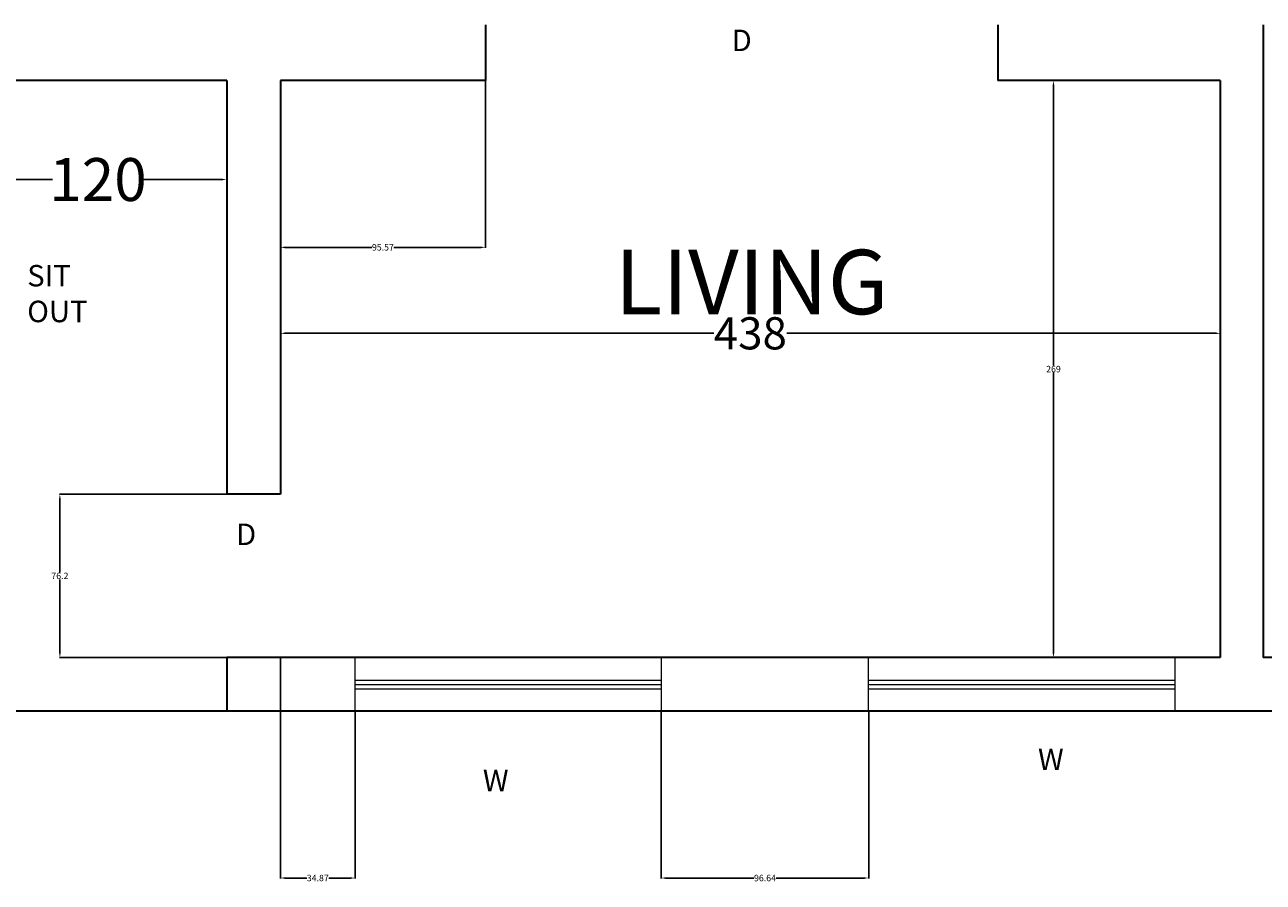
# Model space of a CAD drawing. Units: centimetres. Extents: x -121 to 3851, y -16 to 1180.
# Tile 2 of 16: x 381 to 958, y -16 to 384. Entities that reach past the tile are written whole.
import ezdxf

# ---------------------------------------------------------------- set-up
doc = ezdxf.new("R2010")
doc.units = ezdxf.units.CM
doc.header["$MEASUREMENT"] = 0
for name, color, linetype, lineweight in [('A-ANNO-DIMS', 2, 'Continuous', 18), ('A-ANNO-IDEN', 3, 'Continuous', 13), ('A-AREA-IDEN', 3, 'Continuous', 18), ('A-GLAZ', 4, 'Continuous', 18), ('A-WALL', 7, 'Continuous', 35)]:
    doc.layers.add(name, color=color, linetype=linetype, lineweight=lineweight)
doc.styles.get("Standard").update_dxf_attribs({"font": 'arial.ttf'})
doc.dimstyles.get("Standard").update_dxf_attribs({"dimtxt": 3, "dimasz": 2, "dimexe": 0.18, "dimexo": 0.0625, "dimgap": 0.09, "dimtad": 0, "dimtih": 1, "dimtoh": 1, "dimdec": 0, "dimzin": 0, "dimdsep": 46, "dimtxsty": 'Standard', "dimcen": 0.09, "dimadec": 0, "dimazin": 0, "dimtfac": 1, "dimtdec": 0, "dimtofl": 0, "dimtmove": 0, "dimatfit": 3, "dimfxl": 1, "dimtolj": 1, "dimtzin": 0, "dimarcsym": 0})

# ---------------------------------------------------------------- blocks, each defined once
blk = doc.blocks.new('*D8')
at = {"layer": 'A-ANNO-DIMS', "color": 0, "lineweight": -2, "transparency": 16777216}
for p, q in [((355.04, 281.89), (355.04, 312.04)), ((357.04, 311.86), (393.83, 311.86)), ((473.04, 311.86), (436.25, 311.86)), ((475.04, 281.89), (475.04, 312.04))]:
    blk.add_line(p, q, dxfattribs=at)
at = {"layer": 'A-ANNO-DIMS', "color": 0, "transparency": 16777216}
for points in [[(357.04, 312.19), (357.04, 311.52), (355.04, 311.86)], [(473.04, 312.19), (473.04, 311.52), (475.04, 311.86)]]:
    blk.add_solid(points, dxfattribs=at)
at = {"layer": 'Defpoints', "color": 0, "transparency": 16777216}
for p in [(475.04, 311.86), (355.04, 281.82), (475.04, 281.82)]:
    blk.add_point(p, dxfattribs=at)
at = {"layer": 'A-ANNO-DIMS', "color": 0, "transparency": 16777216, "insert": (415.04, 311.86), "char_height": 3, "attachment_point": 5}
blk.add_mtext('\\A1;{\\H6.66667x;120}', dxfattribs=at)
blk = doc.blocks.new('*D10')
at = {"layer": 'A-ANNO-DIMS', "color": 0, "lineweight": -2, "transparency": 16777216}
for p, q in [((500.04, 198.01), (500.04, 240.36)), ((502.04, 240.18), (702.06, 240.18)), ((936.04, 240.18), (736.02, 240.18)), ((938.04, 198.01), (938.04, 240.36))]:
    blk.add_line(p, q, dxfattribs=at)
at = {"layer": 'A-ANNO-DIMS', "color": 0, "transparency": 16777216}
for points in [[(502.04, 240.52), (502.04, 239.85), (500.04, 240.18)], [(936.04, 240.52), (936.04, 239.85), (938.04, 240.18)]]:
    blk.add_solid(points, dxfattribs=at)
at = {"layer": 'Defpoints', "color": 0, "transparency": 16777216}
for p in [(938.04, 240.18), (500.04, 197.94), (938.04, 197.94)]:
    blk.add_point(p, dxfattribs=at)
at = {"layer": 'A-ANNO-DIMS', "color": 0, "transparency": 16777216, "insert": (719.04, 240.18), "char_height": 3, "attachment_point": 5}
blk.add_mtext('\\A1;{\\H5x;438}', dxfattribs=at)
blk = doc.blocks.new('WIN-143CM')
for p, q in [((0, 14.5), (142.63, 14.5)), ((0, 12.5), (142.63, 12.5)), ((0, 10.5), (142.63, 10.5))]:
    blk.add_line(p, q)
blk.add_lwpolyline([(0, 25), (142.63, 25), (142.63, 0), (0, 0)], close=True)
blk = doc.blocks.new('*D44')
at = {"layer": 'A-ANNO-DIMS', "color": 0, "lineweight": -2, "transparency": 16777216}
for p, q in [((474.98, 165.21), (397.11, 165.21)), ((397.29, 163.21), (397.29, 128.73)), ((397.29, 91.01), (397.29, 125.49)), ((474.98, 89.01), (397.11, 89.01))]:
    blk.add_line(p, q, dxfattribs=at)
at = {"layer": 'A-ANNO-DIMS', "color": 0, "transparency": 16777216}
for points in [[(396.95, 163.21), (397.62, 163.21), (397.29, 165.21)], [(396.95, 91.01), (397.62, 91.01), (397.29, 89.01)]]:
    blk.add_solid(points, dxfattribs=at)
at = {"layer": 'Defpoints', "color": 0, "transparency": 16777216}
for p in [(397.29, 165.21), (475.04, 165.21), (475.04, 89.01)]:
    blk.add_point(p, dxfattribs=at)
at = {"layer": 'A-ANNO-DIMS', "color": 0, "transparency": 16777216, "insert": (397.29, 127.11), "char_height": 3, "attachment_point": 5}
blk.add_mtext('\\A1;76.2', dxfattribs=at)
blk = doc.blocks.new('*D46')
at = {"layer": 'A-ANNO-DIMS', "color": 0, "lineweight": -2, "transparency": 16777216}
for p, q in [((500.04, 357.95), (500.04, 280.08)), ((595.61, 357.95), (595.61, 280.08)), ((502.04, 280.26), (542.67, 280.26)), ((593.61, 280.26), (552.98, 280.26))]:
    blk.add_line(p, q, dxfattribs=at)
at = {"layer": 'A-ANNO-DIMS', "color": 0, "transparency": 16777216}
for points in [[(502.04, 280.6), (502.04, 279.93), (500.04, 280.26)], [(593.61, 280.6), (593.61, 279.93), (595.61, 280.26)]]:
    blk.add_solid(points, dxfattribs=at)
at = {"layer": 'Defpoints', "color": 0, "transparency": 16777216}
for p in [(500.04, 358.01), (595.61, 358.01), (500.04, 280.26)]:
    blk.add_point(p, dxfattribs=at)
at = {"layer": 'A-ANNO-DIMS', "color": 0, "transparency": 16777216, "insert": (547.82, 280.26), "char_height": 3, "attachment_point": 5}
blk.add_mtext('\\A1;95.57', dxfattribs=at)
blk = doc.blocks.new('*D47')
at = {"layer": 'A-ANNO-DIMS', "color": 0, "lineweight": -2, "transparency": 16777216}
for p, q in [((937.98, 358.01), (860.11, 358.01)), ((860.29, 356.01), (860.29, 225.14)), ((860.29, 91.01), (860.29, 221.89)), ((937.98, 89.01), (860.11, 89.01))]:
    blk.add_line(p, q, dxfattribs=at)
at = {"layer": 'A-ANNO-DIMS', "color": 0, "transparency": 16777216}
for points in [[(859.95, 356.01), (860.62, 356.01), (860.29, 358.01)], [(859.95, 91.01), (860.62, 91.01), (860.29, 89.01)]]:
    blk.add_solid(points, dxfattribs=at)
at = {"layer": 'Defpoints', "color": 0, "transparency": 16777216}
for p in [(860.29, 358.01), (938.04, 358.01), (938.04, 89.01)]:
    blk.add_point(p, dxfattribs=at)
at = {"layer": 'A-ANNO-DIMS', "color": 0, "transparency": 16777216, "insert": (860.29, 223.51), "char_height": 3, "attachment_point": 5}
blk.add_mtext('\\A1;269', dxfattribs=at)
blk = doc.blocks.new('*D48')
at = {"layer": 'A-ANNO-DIMS', "color": 0, "lineweight": -2, "transparency": 16777216}
for p, q in [((500.04, 88.95), (500.04, -13.92)), ((534.91, 63.95), (534.91, -13.92)), ((502.04, -13.74), (512.32, -13.74)), ((532.91, -13.74), (522.62, -13.74))]:
    blk.add_line(p, q, dxfattribs=at)
at = {"layer": 'A-ANNO-DIMS', "color": 0, "transparency": 16777216}
for points in [[(502.04, -13.4), (502.04, -14.07), (500.04, -13.74)], [(532.91, -13.4), (532.91, -14.07), (534.91, -13.74)]]:
    blk.add_solid(points, dxfattribs=at)
at = {"layer": 'Defpoints', "color": 0, "transparency": 16777216}
for p in [(500.04, 89.01), (534.91, 64.01), (500.04, -13.74)]:
    blk.add_point(p, dxfattribs=at)
at = {"layer": 'A-ANNO-DIMS', "color": 0, "transparency": 16777216, "insert": (517.47, -13.74), "char_height": 3, "attachment_point": 5}
blk.add_mtext('\\A1;34.87', dxfattribs=at)
blk = doc.blocks.new('*D49')
at = {"layer": 'A-ANNO-DIMS', "color": 0, "lineweight": -2, "transparency": 16777216}
for p, q in [((677.54, 63.95), (677.54, -13.92)), ((774.18, 63.95), (774.18, -13.92)), ((679.54, -13.74), (720.71, -13.74)), ((772.18, -13.74), (731, -13.74))]:
    blk.add_line(p, q, dxfattribs=at)
at = {"layer": 'A-ANNO-DIMS', "color": 0, "transparency": 16777216}
for points in [[(679.54, -13.4), (679.54, -14.07), (677.54, -13.74)], [(772.18, -13.4), (772.18, -14.07), (774.18, -13.74)]]:
    blk.add_solid(points, dxfattribs=at)
at = {"layer": 'Defpoints', "color": 0, "transparency": 16777216}
for p in [(677.54, 64.01), (774.18, 64.01), (774.18, -13.74)]:
    blk.add_point(p, dxfattribs=at)
at = {"layer": 'A-ANNO-DIMS', "color": 0, "transparency": 16777216, "insert": (725.86, -13.74), "char_height": 3, "attachment_point": 5}
blk.add_mtext('\\A1;96.64', dxfattribs=at)

msp = doc.modelspace()

# ---------------------------------------------------------------- linework, layer by layer
at = {"layer": 'A-WALL'}
for p, q in [((595.6084, 384.0141), (595.6084, 358.0141)), ((834.382, 384.0141), (834.382, 358.0141)), ((958.0382, 384.0141), (958.0382, 89.0141)), ((475.0382, 358.0141), (65.0382, 358.0141)), ((475.0382, 358.0141), (475.0382, 165.2103)), ((500.0382, 358.0141), (500.0382, 165.2103)), ((595.6084, 358.0141), (500.0382, 358.0141)), ((938.0382, 358.0141), (834.382, 358.0141)), ((938.0382, 358.0141), (938.0382, 89.0141)), ((500.0382, 165.2103), (475.0382, 165.2103)), ((500.0382, 89.0141), (475.0382, 89.0141)), ((475.0382, 89.0141), (475.0382, 64.0141)), ((938.0382, 89.0141), (500.0382, 89.0141)), ((1396.0382, 89.0141), (958.0382, 89.0141)), ((1421.0382, 64.0141), (65.0382, 64.0141))]:
    msp.add_line(p, q, dxfattribs=at)

# ---------------------------------------------------------------- block references
at = {"layer": 'A-GLAZ'}
for p in [(534.908, 64.014), (774.1757, 64.014)]:
    msp.add_blockref('WIN-143CM', p, dxfattribs=at)

# ---------------------------------------------------------------- texts
at = {"layer": 'A-ANNO-IDEN', "char_height": 10, "attachment_point": 1}
for s, insert in [('D', (710.312, 381.728)), ('D', (479.3761, 151.4737)), ('W', (853.0789, 46.5447)), ('W', (594.4052, 36.7331))]:
    msp.add_mtext_dynamic_manual_height_columns(s, width=55.718495, gutter_width=1, heights=[0], dxfattribs=dict(at, insert=insert))
at = {"layer": 'A-AREA-IDEN', "attachment_point": 1}
for s, width, insert, char_height in [('LIVING', 354.505754, (655.815, 279.0974), 30), ('SIT OUT', 31.141092, (382.0658, 272.0373), 10)]:
    msp.add_mtext_dynamic_manual_height_columns(s, width=width, gutter_width=1, heights=[0], dxfattribs=dict(at, insert=insert, char_height=char_height))

# ---------------------------------------------------------------- dimensions: what is measured, and where the dimension line sits
at = {"layer": 'A-ANNO-DIMS'}
for base, p1, p2, angle, override, picture, middle in [((500.0382, 280.2641), (595.6084, 358.0141), (500.0382, 358.0141), 180, {"dimdec": 2, "dimlfac": 1, "dimrnd": 0, "dimzin": 0, "dimdsep": 46, "dimlunit": 2}, '*D46', (547.8233, 280.2641)), ((860.2882, 358.0141), (938.0382, 89.0141), (938.0382, 358.0141), 90, {"dimdec": 0, "dimlfac": 1, "dimrnd": 0, "dimzin": 0, "dimdsep": 46, "dimlunit": 2}, '*D47', (860.2882, 223.5141)), ((397.2882, 165.2103), (475.0382, 89.0141), (475.0382, 165.2103), 90, {"dimdec": 1, "dimlfac": 1, "dimrnd": 0, "dimzin": 0, "dimdsep": 46, "dimlunit": 2}, '*D44', (397.2882, 127.1122))]:
    dim = msp.add_linear_dim(base=base, p1=p1, p2=p2, angle=angle, dimstyle='Standard', override=override, dxfattribs=at)
    dim.commit()
    dim.dimension.update_dxf_attribs({"geometry": picture, "text_midpoint": middle})
for base, p1, p2, text, picture, middle in [((475.0382, 311.8567), (355.0382, 281.8249), (475.0382, 281.8249), '{\\H6.66667x;<>}', '*D8', (415.0382, 311.8567)), ((938.0382, 240.1848), (500.0382, 197.9428), (938.0382, 197.9428), '{\\H5x;<>}', '*D10', (719.0382, 240.1848))]:
    dim = msp.add_linear_dim(base=base, p1=p1, p2=p2, text=text, dimstyle='Standard', override={"dimclrd": 0, "dimclre": 0, "dimclrt": 0}, dxfattribs=at)
    dim.commit()
    dim.dimension.update_dxf_attribs({"geometry": picture, "text_midpoint": middle})
for base, p1, p2, picture, middle in [((500.0382, -13.7359), (534.9081, 64.0141), (500.0382, 89.0141), '*D48', (517.4731, -13.7359)), ((774.1758, -13.7359), (677.5363, 64.0141), (774.1758, 64.0141), '*D49', (725.856, -13.7359))]:
    dim = msp.add_linear_dim(base=base, p1=p1, p2=p2, dimstyle='Standard', override={"dimdec": 2, "dimlfac": 1, "dimrnd": 0, "dimzin": 0, "dimdsep": 46, "dimlunit": 2}, dxfattribs=at)
    dim.commit()
    dim.dimension.update_dxf_attribs({"geometry": picture, "text_midpoint": middle})

doc.saveas('drawing.dxf')
